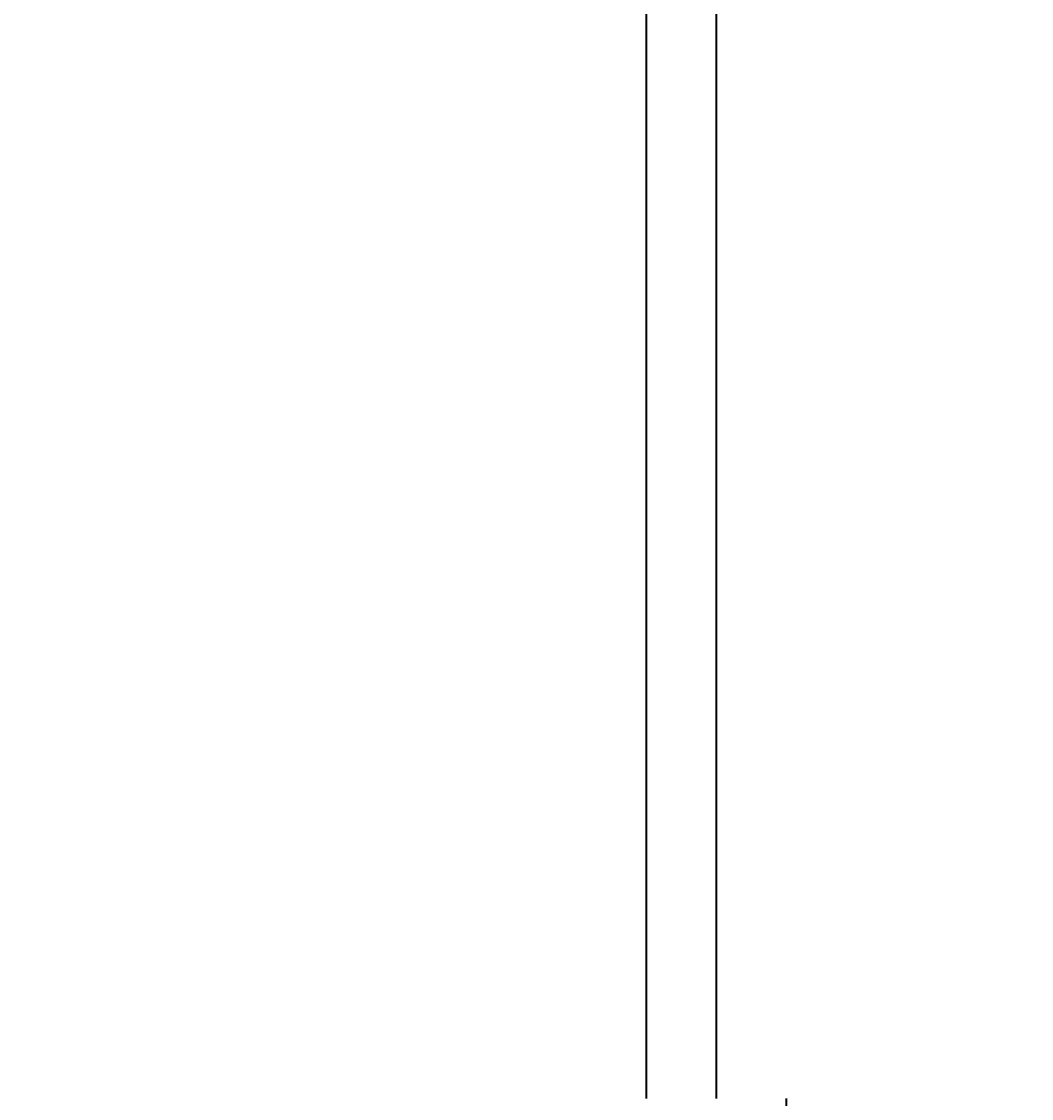
# Model space of a CAD drawing. Units: inches. Extents: x 4159 to 4826, y 299 to 1026.
# Tile 5 of 37: x 4268 to 4354, y 401 to 494. Entities that reach past the tile are written whole.
import ezdxf

# ---------------------------------------------------------------- set-up
doc = ezdxf.new("R2010")
doc.units = ezdxf.units.IN
doc.layers.add('A-ANNO-DIMS', color=2, linetype='Continuous', lineweight=18)
doc.layers.add('A-WALL', color=7, linetype='Continuous', lineweight=35)
doc.styles.get("Standard").update_dxf_attribs({"font": 'arial.ttf'})
doc.dimstyles.get("Standard").update_dxf_attribs({"dimtxt": 0.18, "dimasz": 0.18, "dimexe": 0.18, "dimexo": 0.0625, "dimgap": 0.09, "dimtad": 0, "dimtih": 1, "dimtoh": 1, "dimdec": 4, "dimzin": 0, "dimdsep": 46, "dimtxsty": 'Standard', "dimcen": 0.09, "dimadec": 0, "dimazin": 0, "dimtfac": 1, "dimtdec": 4, "dimtofl": 0, "dimtmove": 0, "dimatfit": 3, "dimfxl": 1, "dimtolj": 1, "dimtzin": 0, "dimarcsym": 0})

# ---------------------------------------------------------------- blocks, each defined once
blk = doc.blocks.new('*D44')
at = {"layer": 'A-ANNO-DIMS', "color": 0, "lineweight": -2, "transparency": 16777216}
for p, q in [((4287.263, 963.093), (4158.88, 963.093)), ((4159.06, 962.913), (4159.06, 647.826)), ((4159.06, 332.375), (4159.06, 647.462)), ((4447.248, 332.195), (4158.88, 332.195))]:
    blk.add_line(p, q, dxfattribs=at)
at = {"layer": 'A-ANNO-DIMS', "color": 0, "transparency": 16777216}
for points in [[(4159.03, 962.913), (4159.09, 962.913), (4159.06, 963.093)], [(4159.03, 332.375), (4159.09, 332.375), (4159.06, 332.195)]]:
    blk.add_solid(points, dxfattribs=at)
at = {"layer": 'Defpoints', "color": 0, "transparency": 16777216}
for p in [(4287.326, 963.093), (4159.06, 332.195), (4447.31, 332.195)]:
    blk.add_point(p, dxfattribs=at)
at = {"layer": 'A-ANNO-DIMS', "color": 0, "transparency": 16777216, "insert": (4159.06, 647.644), "char_height": 0.18, "attachment_point": 5}
blk.add_mtext('\\A1;630.9', dxfattribs=at)

msp = doc.modelspace()

# ---------------------------------------------------------------- linework, layer by layer
at = {"layer": 'A-WALL'}
for p, q in [((4321.31, 533.254), (4321.31, 401.254)), ((4327.31, 533.254), (4327.31, 401.254)), ((4333.31, 401.254), (4333.31, 392.254))]:
    msp.add_line(p, q, dxfattribs=at)

# ---------------------------------------------------------------- dimensions: what is measured, and where the dimension line sits
at = {"layer": 'A-ANNO-DIMS'}
dim = msp.add_linear_dim(base=(4159.06, 332.195), p1=(4287.326, 963.093), p2=(4447.31, 332.195), angle=90, dimstyle='Standard', override={"dimdec": 1, "dimlfac": 1, "dimrnd": 0, "dimzin": 0, "dimdsep": 46, "dimlunit": 2}, dxfattribs=at)
dim.commit()
dim.dimension.update_dxf_attribs({"geometry": '*D44', "text_midpoint": (4159.06, 647.644)})

doc.saveas('drawing.dxf')
